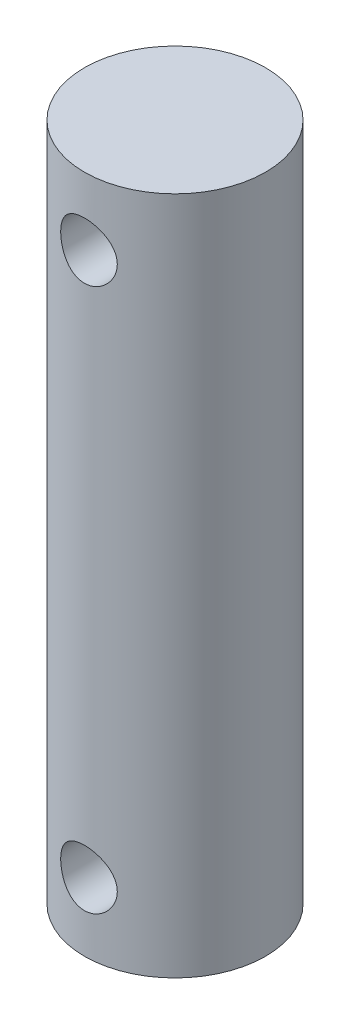
ISO-10303-21;
HEADER;
FILE_DESCRIPTION(('STEP AP214'),'2;1');
FILE_NAME('part.step','',(''),(''),'','','');
FILE_SCHEMA(('AUTOMOTIVE_DESIGN { 1 0 10303 214 1 1 1 1 }'));
ENDSEC;
DATA;
#1=APPLICATION_CONTEXT('core data for automotive mechanical design processes');
#2=APPLICATION_PROTOCOL_DEFINITION('international standard','automotive_design',2000,#1);
#3=PRODUCT_CONTEXT('',#1,'mechanical');
#4=PRODUCT('Part','Part','',(#3));
#5=PRODUCT_RELATED_PRODUCT_CATEGORY('part','',(#4));
#6=PRODUCT_DEFINITION_FORMATION('','',#4);
#7=PRODUCT_DEFINITION_CONTEXT('part definition',#1,'design');
#8=PRODUCT_DEFINITION('design','',#6,#7);
#9=PRODUCT_DEFINITION_SHAPE('','',#8);
#10=(LENGTH_UNIT() NAMED_UNIT(*) SI_UNIT(.MILLI.,.METRE.));
#11=(NAMED_UNIT(*) PLANE_ANGLE_UNIT() SI_UNIT($,.RADIAN.));
#12=(NAMED_UNIT(*) SI_UNIT($,.STERADIAN.) SOLID_ANGLE_UNIT());
#13=UNCERTAINTY_MEASURE_WITH_UNIT(LENGTH_MEASURE(1.E-05),#10,'distance_accuracy_value','');
#14=(GEOMETRIC_REPRESENTATION_CONTEXT(3) GLOBAL_UNCERTAINTY_ASSIGNED_CONTEXT((#13)) GLOBAL_UNIT_ASSIGNED_CONTEXT((#10,
#11,#12)) REPRESENTATION_CONTEXT('',''));
#15=CARTESIAN_POINT('',(0.,0.,0.));
#16=DIRECTION('',(0.,0.,1.));
#17=DIRECTION('',(1.,0.,0.));
#18=AXIS2_PLACEMENT_3D('',#15,#16,#17);
#19=CARTESIAN_POINT('',(0.,30.,0.));
#20=DIRECTION('',(0.,-1.,0.));
#21=DIRECTION('',(0.,0.,-1.));
#22=AXIS2_PLACEMENT_3D('',#19,#20,#21);
#23=CYLINDRICAL_SURFACE('',#22,8.);
#24=CARTESIAN_POINT('',(0.,26.5,-8.));
#25=CARTESIAN_POINT('',(-0.136878370349093,26.4999991068248,-7.9999993175598));
#26=CARTESIAN_POINT('',(-0.273766105005718,26.4887215461111,-7.99645389969682));
#27=CARTESIAN_POINT('',(-0.543538419176897,26.4440275169215,-7.98265788177613));
#28=CARTESIAN_POINT('',(-0.676422085451815,26.4106060372713,-7.97240576399719));
#29=CARTESIAN_POINT('',(-0.934257087301612,26.3228612576085,-7.94631631395819));
#30=CARTESIAN_POINT('',(-1.05922035397161,26.2685703106941,-7.9304876299805));
#31=CARTESIAN_POINT('',(-1.29826960469292,26.1407653646433,-7.89487938322185));
#32=CARTESIAN_POINT('',(-1.41235387088977,26.0672483364388,-7.8750991979981));
#33=CARTESIAN_POINT('',(-1.62993066990456,25.9006880159653,-7.83300427480565));
#34=CARTESIAN_POINT('',(-1.73304005631332,25.8071582298779,-7.81063431853978));
#35=CARTESIAN_POINT('',(-1.92239476407399,25.6042632151729,-7.76620092748417));
#36=CARTESIAN_POINT('',(-2.00863694579739,25.4948950450109,-7.74413755046915));
#37=CARTESIAN_POINT('',(-2.16388672966227,25.2601108723838,-7.70222289396344));
#38=CARTESIAN_POINT('',(-2.23241568300258,25.1343650449456,-7.68243976603591));
#39=CARTESIAN_POINT('',(-2.34719482153343,24.8724153700363,-7.64815603598469));
#40=CARTESIAN_POINT('',(-2.39345087543889,24.7362142884121,-7.63365404257377));
#41=CARTESIAN_POINT('',(-2.46096919860067,24.4615438450959,-7.61215213969001));
#42=CARTESIAN_POINT('',(-2.48294220015729,24.3232663127223,-7.60493945859016));
#43=CARTESIAN_POINT('',(-2.50349110073976,24.0448137621762,-7.59820110281901));
#44=CARTESIAN_POINT('',(-2.50207321991544,23.9046392583567,-7.59867338454668));
#45=CARTESIAN_POINT('',(-2.47643649465479,23.632251079462,-7.60706378150876));
#46=CARTESIAN_POINT('',(-2.45312115738766,23.4999417482769,-7.61468683491897));
#47=CARTESIAN_POINT('',(-2.38581626711252,23.2412156869253,-7.63604051304978));
#48=CARTESIAN_POINT('',(-2.34182451689101,23.1147995845824,-7.6497717868623));
#49=CARTESIAN_POINT('',(-2.23377749362554,22.8692961111347,-7.68202088028593));
#50=CARTESIAN_POINT('',(-2.16943851324164,22.750342778616,-7.70060569321649));
#51=CARTESIAN_POINT('',(-2.02272041475696,22.5246244642418,-7.7404371316014));
#52=CARTESIAN_POINT('',(-1.94033661043155,22.4178626594926,-7.76168444789102));
#53=CARTESIAN_POINT('',(-1.75543390836425,22.214450113166,-7.80563055600986));
#54=CARTESIAN_POINT('',(-1.65216914118563,22.1184808844406,-7.82835139211391));
#55=CARTESIAN_POINT('',(-1.43072881619106,21.9450562128406,-7.87183141519161));
#56=CARTESIAN_POINT('',(-1.31255215469804,21.8676021415616,-7.89259045676745));
#57=CARTESIAN_POINT('',(-1.06332922093091,21.7329446227975,-7.93002589780382));
#58=CARTESIAN_POINT('',(-0.932189813838561,21.6759037290721,-7.94666921296415));
#59=CARTESIAN_POINT('',(-0.661535955565289,21.5848939982969,-7.97375911657108));
#60=CARTESIAN_POINT('',(-0.522024061449216,21.5509181555232,-7.98420758650304));
#61=CARTESIAN_POINT('',(-0.244370314580689,21.508163914842,-7.99742778790027));
#62=CARTESIAN_POINT('',(-0.106383697577685,21.498462912813,-8.00048045790873));
#63=CARTESIAN_POINT('',(0.169260611465172,21.5019324532747,-7.99939599461967));
#64=CARTESIAN_POINT('',(0.306918348613018,21.5150996546452,-7.9952599116227));
#65=CARTESIAN_POINT('',(0.574438665951698,21.5631911852128,-7.98044727539523));
#66=CARTESIAN_POINT('',(0.704409956841874,21.597566535225,-7.96993586221374));
#67=CARTESIAN_POINT('',(0.956703857722754,21.6864287047334,-7.94360242758579));
#68=CARTESIAN_POINT('',(1.07902552089812,21.74091800805,-7.92777975028687));
#69=CARTESIAN_POINT('',(1.31586481334438,21.8699464330974,-7.89197085518848));
#70=CARTESIAN_POINT('',(1.43011947957558,21.9449419749936,-7.87189253635335));
#71=CARTESIAN_POINT('',(1.64473170192052,22.1123064202348,-7.82986820006859));
#72=CARTESIAN_POINT('',(1.7450854760879,22.2046800354893,-7.80792167695774));
#73=CARTESIAN_POINT('',(1.93317492583804,22.4085177801042,-7.76353989766283));
#74=CARTESIAN_POINT('',(2.02025304679063,22.5205933274784,-7.74111973412882));
#75=CARTESIAN_POINT('',(2.17442500490303,22.7582532327535,-7.69923894191212));
#76=CARTESIAN_POINT('',(2.24151915946859,22.883837376054,-7.67977826622621));
#77=CARTESIAN_POINT('',(2.35340166961085,23.144690345741,-7.64623564661738));
#78=CARTESIAN_POINT('',(2.39827639112025,23.2799192988714,-7.63213292713749));
#79=CARTESIAN_POINT('',(2.4644578863618,23.5565449864972,-7.6110234168862));
#80=CARTESIAN_POINT('',(2.48577362827989,23.6979393526871,-7.60401392602456));
#81=CARTESIAN_POINT('',(2.50358812316251,23.9760081751609,-7.59816585427753));
#82=CARTESIAN_POINT('',(2.50116559243271,24.1126069076948,-7.59897209200284));
#83=CARTESIAN_POINT('',(2.47417636257668,24.3833491698839,-7.60780180751807));
#84=CARTESIAN_POINT('',(2.44961069645024,24.5174928137735,-7.61582494863208));
#85=CARTESIAN_POINT('',(2.37975459827235,24.7775880791838,-7.6379362836678));
#86=CARTESIAN_POINT('',(2.33477284812017,24.9036308821867,-7.65193396380514));
#87=CARTESIAN_POINT('',(2.22560454669999,25.146480827068,-7.68439408509128));
#88=CARTESIAN_POINT('',(2.16141408888474,25.2632860841568,-7.70285743429343));
#89=CARTESIAN_POINT('',(2.01271350026987,25.4892919408796,-7.74306974067005));
#90=CARTESIAN_POINT('',(1.92750667048265,25.5980162590005,-7.76491897845913));
#91=CARTESIAN_POINT('',(1.7404179928096,25.799972656224,-7.8089799764242));
#92=CARTESIAN_POINT('',(1.63853168468878,25.8932005779821,-7.83119183213309));
#93=CARTESIAN_POINT('',(1.41697332564669,26.0645650767259,-7.87434543904947));
#94=CARTESIAN_POINT('',(1.29682914897477,26.1421094728999,-7.89522203461346));
#95=CARTESIAN_POINT('',(1.0445582760273,26.2757978302789,-7.93253538593756));
#96=CARTESIAN_POINT('',(0.912436315590895,26.3319502042837,-7.94897388631644));
#97=CARTESIAN_POINT('',(0.651495270747956,26.4171827352169,-7.97441301466941));
#98=CARTESIAN_POINT('',(0.523340674225092,26.4481497346107,-7.98392481612283));
#99=CARTESIAN_POINT('',(0.263459790880495,26.4895567199354,-7.99671800680967));
#100=CARTESIAN_POINT('',(0.131734232279349,26.500000859608,-8.00000065679286));
#101=CARTESIAN_POINT('',(0.,26.5,-8.));
#102=B_SPLINE_CURVE_WITH_KNOTS('',3,(#24,#25,#26,#27,#28,#29,#30,#31,#32,#33,#34,#35,#36,#37,
#38,#39,#40,#41,#42,#43,#44,#45,#46,#47,#48,#49,#50,#51,#52,#53,#54,#55,#56,#57,#58,#59,#60,#61,
#62,#63,#64,#65,#66,#67,#68,#69,#70,#71,#72,#73,#74,#75,#76,#77,#78,#79,#80,#81,#82,#83,#84,#85,
#86,#87,#88,#89,#90,#91,#92,#93,#94,#95,#96,#97,#98,#99,#100,#101),.UNSPECIFIED.,.T.,.F.,(4,2,2,
2,2,2,2,2,2,2,2,2,2,2,2,2,2,2,2,2,2,2,2,2,2,2,2,2,2,2,2,2,2,2,2,2,2,2,4),(0.,0.41015089886502,
0.820394646698132,1.23000495840487,1.63967984311678,2.06075644390316,2.48191134862552,
2.91347542494988,3.34492572559054,3.7633830033442,4.18172900590277,4.58353834844338,
4.98539039958126,5.39311285441091,5.80094132020717,6.22733494559201,6.65376014826606,
7.0835092137954,7.51312768989108,7.92615137096475,8.33911471298726,8.74181253445744,
9.14456010069,9.55712649476687,9.96980491418519,10.3988355742628,10.8278594196742,
11.2552023150671,11.6823824779468,12.0902440696666,12.4980866352126,12.8999582681244,
13.3019116867944,13.7195902803182,14.1373807476578,14.5688133627192,15.0000761335177,
15.3948927332218,15.7896294154519),.UNSPECIFIED.);
#103=CARTESIAN_POINT('',(0.,26.5,-8.));
#104=VERTEX_POINT('',#103);
#105=EDGE_CURVE('E10',#104,#104,#102,.T.);
#106=ORIENTED_EDGE('',*,*,#105,.T.);
#107=EDGE_LOOP('',(#106));
#108=FACE_BOUND('',#107,.T.);
#109=CARTESIAN_POINT('',(2.5,24.,7.59934207678533));
#110=CARTESIAN_POINT('',(2.49999907560094,23.8633059277813,7.59934291923872));
#111=CARTESIAN_POINT('',(2.48875077582989,23.7266024625936,7.60307063010085));
#112=CARTESIAN_POINT('',(2.44418350802654,23.4572116782444,7.61751277997754));
#113=CARTESIAN_POINT('',(2.4108585756503,23.3245254545357,7.62822910706272));
#114=CARTESIAN_POINT('',(2.32339576447118,23.067110196136,7.65531877671919));
#115=CARTESIAN_POINT('',(2.26929471473354,22.9423675337886,7.67168210388634));
#116=CARTESIAN_POINT('',(2.14193828346314,22.703694608272,7.70820812437377));
#117=CARTESIAN_POINT('',(2.06867951811264,22.5897662600798,7.72837148871681));
#118=CARTESIAN_POINT('',(1.90239214124459,22.372042265013,7.7710025533724));
#119=CARTESIAN_POINT('',(1.8088187994408,22.268672781128,7.79352246769561));
#120=CARTESIAN_POINT('',(1.60572409291099,22.0788079735816,7.83788491720671));
#121=CARTESIAN_POINT('',(1.49620050503713,21.9923150061103,7.85972735745255));
#122=CARTESIAN_POINT('',(1.26125182498672,21.8367778739775,7.90087106780156));
#123=CARTESIAN_POINT('',(1.13552311304019,21.7681725923371,7.9201036912556));
#124=CARTESIAN_POINT('',(0.873608465706806,21.6532479002889,7.95325103666038));
#125=CARTESIAN_POINT('',(0.737424996974103,21.6069232517008,7.9671670083984));
#126=CARTESIAN_POINT('',(0.462928713932197,21.5392977438059,7.98774351641724));
#127=CARTESIAN_POINT('',(0.324811430936433,21.5172685004243,7.99461477968283));
#128=CARTESIAN_POINT('',(0.0466816279690395,21.496551307125,8.00107191752033));
#129=CARTESIAN_POINT('',(-0.0933304539461723,21.4978580512823,8.00065944820141));
#130=CARTESIAN_POINT('',(-0.366148960709462,21.5232965831719,7.99274232265063));
#131=CARTESIAN_POINT('',(-0.499037268628064,21.546638767026,7.98548301944274));
#132=CARTESIAN_POINT('',(-0.75890612669556,21.614189980086,7.9649896512175));
#133=CARTESIAN_POINT('',(-0.88588629096247,21.6584003701733,7.95175519654419));
#134=CARTESIAN_POINT('',(-1.13215620630948,21.7669403781496,7.92046919458913));
#135=CARTESIAN_POINT('',(-1.25133281124535,21.8315096171255,7.90236067233341));
#136=CARTESIAN_POINT('',(-1.47740502230436,21.9787421994097,7.86323445907697));
#137=CARTESIAN_POINT('',(-1.58429751241882,22.0614101182777,7.84221603291309));
#138=CARTESIAN_POINT('',(-1.78747539690657,22.2465472696004,7.79847341467064));
#139=CARTESIAN_POINT('',(-1.88313309818382,22.3496981376742,7.77571463969686));
#140=CARTESIAN_POINT('',(-2.05597948519529,22.5707902036571,7.73181230889308));
#141=CARTESIAN_POINT('',(-2.13316599552377,22.6887331411807,7.71066894351396));
#142=CARTESIAN_POINT('',(-2.26760930038169,22.9378349376951,7.6722169326579));
#143=CARTESIAN_POINT('',(-2.32463361399527,23.0691268179819,7.65495380588195));
#144=CARTESIAN_POINT('',(-2.41556691891091,23.340118983684,7.62675090557699));
#145=CARTESIAN_POINT('',(-2.44948421530003,23.4798162283887,7.61580886035023));
#146=CARTESIAN_POINT('',(-2.4920297037281,23.7576399051543,7.60199126814082));
#147=CARTESIAN_POINT('',(-2.50161908707794,23.8956039924703,7.59880932787512));
#148=CARTESIAN_POINT('',(-2.49793488996242,24.1711794829903,7.6000215491985));
#149=CARTESIAN_POINT('',(-2.48466484222813,24.3087909373993,7.60441454014633));
#150=CARTESIAN_POINT('',(-2.43649747026382,24.5756165933048,7.61997914967833));
#151=CARTESIAN_POINT('',(-2.40223662321101,24.7049585481484,7.63095108204023));
#152=CARTESIAN_POINT('',(-2.31380747322029,24.9560435839917,7.65822574662762));
#153=CARTESIAN_POINT('',(-2.25963592342302,25.0777854218423,7.67452934824624));
#154=CARTESIAN_POINT('',(-2.13115021311757,25.3140782195436,7.71121079306468));
#155=CARTESIAN_POINT('',(-2.05630294977117,25.4283228311856,7.73169206979508));
#156=CARTESIAN_POINT('',(-1.8892128173596,25.6429806927238,7.77420697945615));
#157=CARTESIAN_POINT('',(-1.79696542938156,25.7433903378507,7.79624101471394));
#158=CARTESIAN_POINT('',(-1.59314589550721,25.9318207318256,7.84048375125371));
#159=CARTESIAN_POINT('',(-1.48093129957704,26.0191555722797,7.86266184571362));
#160=CARTESIAN_POINT('',(-1.24290309130279,26.1737820866425,7.90378119687353));
#161=CARTESIAN_POINT('',(-1.11709010221725,26.2410746786221,7.92272260181891));
#162=CARTESIAN_POINT('',(-0.856211046663665,26.3530611249434,7.95512623857025));
#163=CARTESIAN_POINT('',(-0.721220368567513,26.3979185756874,7.968627991224));
#164=CARTESIAN_POINT('',(-0.445114508112781,26.4641450771794,7.98880485297152));
#165=CARTESIAN_POINT('',(-0.304001256680715,26.485521478167,7.99548209828555));
#166=CARTESIAN_POINT('',(-0.0259698732978004,26.5035820034992,8.00111606808923));
#167=CARTESIAN_POINT('',(0.110878383893042,26.5012569003415,8.0003825881478));
#168=CARTESIAN_POINT('',(0.382146443846494,26.4743763779026,7.99201956162097));
#169=CARTESIAN_POINT('',(0.516566404359135,26.4498224080161,7.98439046465238));
#170=CARTESIAN_POINT('',(0.777510236961581,26.3798119815555,7.96319141689591));
#171=CARTESIAN_POINT('',(0.904111836898961,26.3346207843093,7.9496969592041));
#172=CARTESIAN_POINT('',(1.14799685100018,26.224858345583,7.918158911759));
#173=CARTESIAN_POINT('',(1.26527866254896,26.1602837800531,7.90011454182716));
#174=CARTESIAN_POINT('',(1.49152338993938,26.0110544833111,7.86059793766752));
#175=CARTESIAN_POINT('',(1.60006921410622,25.9257929550721,7.83903019501924));
#176=CARTESIAN_POINT('',(1.80164158279864,25.7386802211131,7.79517473094122));
#177=CARTESIAN_POINT('',(1.89466346700832,25.6368240517212,7.77288679569653));
#178=CARTESIAN_POINT('',(2.06565731822505,25.4153685603178,7.72923785154876));
#179=CARTESIAN_POINT('',(2.14302855989422,25.2952931937668,7.70793201726912));
#180=CARTESIAN_POINT('',(2.27640941497043,25.0432037594617,7.66960250559062));
#181=CARTESIAN_POINT('',(2.33242766807092,24.9111945470995,7.65257709722773));
#182=CARTESIAN_POINT('',(2.41742360871585,24.6505547653707,7.62613120880655));
#183=CARTESIAN_POINT('',(2.44829879675747,24.5225949050969,7.61618630087498));
#184=CARTESIAN_POINT('',(2.48958491632199,24.263092335807,7.60279212964797));
#185=CARTESIAN_POINT('',(2.50000088961557,24.131550517597,7.59934126603196));
#186=CARTESIAN_POINT('',(2.5,24.,7.59934207678533));
#187=B_SPLINE_CURVE_WITH_KNOTS('',3,(#109,#110,#111,#112,#113,#114,#115,#116,#117,#118,#119,
#120,#121,#122,#123,#124,#125,#126,#127,#128,#129,#130,#131,#132,#133,#134,#135,#136,#137,#138,
#139,#140,#141,#142,#143,#144,#145,#146,#147,#148,#149,#150,#151,#152,#153,#154,#155,#156,#157,
#158,#159,#160,#161,#162,#163,#164,#165,#166,#167,#168,#169,#170,#171,#172,#173,#174,#175,#176,
#177,#178,#179,#180,#181,#182,#183,#184,#185,#186),.UNSPECIFIED.,.T.,.F.,(4,2,2,2,2,2,2,2,2,2,2,
2,2,2,2,2,2,2,2,2,2,2,2,2,2,2,2,2,2,2,2,2,2,2,2,2,2,2,4),(0.,0.409596275096981,
0.819303254119471,1.22828728823716,1.6373436098499,2.05914161101677,2.48099845882246,
2.91239643927466,3.34369294835844,3.76167445671067,4.17956092943549,4.58301965939501,
4.98650470380186,5.39492809216818,5.80345485426375,6.22900677874668,6.65460879707552,
7.08496941871143,7.51517527910369,7.92809866580735,8.34095824443042,8.7418794409359,
9.14286604511284,9.55535226624085,9.96794576028624,10.3976387562789,10.8273120663904,
11.2538047858686,11.6801639628603,12.0887760488391,12.4973614938948,12.9008369303438,
13.3043815982817,13.7216138621529,14.1389711554924,14.5701559100827,15.0011660161251,
15.3954470874764,15.7896309838242),.UNSPECIFIED.);
#188=CARTESIAN_POINT('',(2.5,24.,7.59934207678533));
#189=VERTEX_POINT('',#188);
#190=EDGE_CURVE('E48',#189,#189,#187,.T.);
#191=ORIENTED_EDGE('',*,*,#190,.T.);
#192=EDGE_LOOP('',(#191));
#193=FACE_BOUND('',#192,.T.);
#194=CARTESIAN_POINT('',(0.,-21.5,-8.));
#195=CARTESIAN_POINT('',(-0.136878370349093,-21.5000008931752,-7.9999993175598));
#196=CARTESIAN_POINT('',(-0.273766105005718,-21.5112784538889,-7.99645389969682));
#197=CARTESIAN_POINT('',(-0.543538419176897,-21.5559724830785,-7.98265788177613));
#198=CARTESIAN_POINT('',(-0.676422085451815,-21.5893939627287,-7.97240576399719));
#199=CARTESIAN_POINT('',(-0.934257087301612,-21.6771387423915,-7.94631631395819));
#200=CARTESIAN_POINT('',(-1.05922035397161,-21.7314296893059,-7.9304876299805));
#201=CARTESIAN_POINT('',(-1.29826960469292,-21.8592346353567,-7.89487938322185));
#202=CARTESIAN_POINT('',(-1.41235387088977,-21.9327516635612,-7.8750991979981));
#203=CARTESIAN_POINT('',(-1.62993066990456,-22.0993119840347,-7.83300427480565));
#204=CARTESIAN_POINT('',(-1.73304005631332,-22.1928417701221,-7.81063431853978));
#205=CARTESIAN_POINT('',(-1.92239476407399,-22.3957367848271,-7.76620092748417));
#206=CARTESIAN_POINT('',(-2.00863694579739,-22.5051049549891,-7.74413755046915));
#207=CARTESIAN_POINT('',(-2.16388672966227,-22.7398891276162,-7.70222289396344));
#208=CARTESIAN_POINT('',(-2.23241568300257,-22.8656349550544,-7.68243976603591));
#209=CARTESIAN_POINT('',(-2.34719482153343,-23.1275846299637,-7.64815603598469));
#210=CARTESIAN_POINT('',(-2.39345087543889,-23.2637857115879,-7.63365404257377));
#211=CARTESIAN_POINT('',(-2.46096919860067,-23.5384561549041,-7.61215213969001));
#212=CARTESIAN_POINT('',(-2.48294220015729,-23.6767336872777,-7.60493945859016));
#213=CARTESIAN_POINT('',(-2.50349110073976,-23.9551862378238,-7.59820110281901));
#214=CARTESIAN_POINT('',(-2.50207321991544,-24.0953607416433,-7.59867338454668));
#215=CARTESIAN_POINT('',(-2.47643649465479,-24.367748920538,-7.60706378150876));
#216=CARTESIAN_POINT('',(-2.45312115738766,-24.5000582517231,-7.61468683491897));
#217=CARTESIAN_POINT('',(-2.38581626711252,-24.7587843130747,-7.63604051304978));
#218=CARTESIAN_POINT('',(-2.34182451689101,-24.8852004154176,-7.6497717868623));
#219=CARTESIAN_POINT('',(-2.23377749362554,-25.1307038888653,-7.68202088028593));
#220=CARTESIAN_POINT('',(-2.16943851324164,-25.249657221384,-7.70060569321649));
#221=CARTESIAN_POINT('',(-2.02272041475696,-25.4753755357583,-7.7404371316014));
#222=CARTESIAN_POINT('',(-1.94033661043155,-25.5821373405074,-7.76168444789102));
#223=CARTESIAN_POINT('',(-1.75543390836425,-25.785549886834,-7.80563055600986));
#224=CARTESIAN_POINT('',(-1.65216914118563,-25.8815191155594,-7.82835139211391));
#225=CARTESIAN_POINT('',(-1.43072881619106,-26.0549437871594,-7.87183141519161));
#226=CARTESIAN_POINT('',(-1.31255215469804,-26.1323978584384,-7.89259045676745));
#227=CARTESIAN_POINT('',(-1.06332922093091,-26.2670553772026,-7.93002589780382));
#228=CARTESIAN_POINT('',(-0.932189813838561,-26.3240962709279,-7.94666921296415));
#229=CARTESIAN_POINT('',(-0.661535955565289,-26.4151060017031,-7.97375911657108));
#230=CARTESIAN_POINT('',(-0.522024061449216,-26.4490818444768,-7.98420758650304));
#231=CARTESIAN_POINT('',(-0.244370314580689,-26.491836085158,-7.99742778790027));
#232=CARTESIAN_POINT('',(-0.106383697577685,-26.5015370871871,-8.00048045790873));
#233=CARTESIAN_POINT('',(0.169260611465172,-26.4980675467253,-7.99939599461967));
#234=CARTESIAN_POINT('',(0.306918348613018,-26.4849003453548,-7.9952599116227));
#235=CARTESIAN_POINT('',(0.574438665951697,-26.4368088147872,-7.98044727539523));
#236=CARTESIAN_POINT('',(0.704409956841873,-26.402433464775,-7.96993586221374));
#237=CARTESIAN_POINT('',(0.956703857722753,-26.3135712952666,-7.94360242758579));
#238=CARTESIAN_POINT('',(1.07902552089812,-26.25908199195,-7.92777975028687));
#239=CARTESIAN_POINT('',(1.31586481334438,-26.1300535669026,-7.89197085518848));
#240=CARTESIAN_POINT('',(1.43011947957558,-26.0550580250064,-7.87189253635335));
#241=CARTESIAN_POINT('',(1.64473170192052,-25.8876935797652,-7.82986820006859));
#242=CARTESIAN_POINT('',(1.7450854760879,-25.7953199645107,-7.80792167695774));
#243=CARTESIAN_POINT('',(1.93317492583804,-25.5914822198958,-7.76353989766283));
#244=CARTESIAN_POINT('',(2.02025304679062,-25.4794066725216,-7.74111973412883));
#245=CARTESIAN_POINT('',(2.17442500490303,-25.2417467672465,-7.69923894191212));
#246=CARTESIAN_POINT('',(2.24151915946859,-25.116162623946,-7.67977826622621));
#247=CARTESIAN_POINT('',(2.35340166961084,-24.855309654259,-7.64623564661738));
#248=CARTESIAN_POINT('',(2.39827639112025,-24.7200807011286,-7.63213292713749));
#249=CARTESIAN_POINT('',(2.4644578863618,-24.4434550135028,-7.6110234168862));
#250=CARTESIAN_POINT('',(2.48577362827989,-24.3020606473129,-7.60401392602456));
#251=CARTESIAN_POINT('',(2.50358812316251,-24.0239918248391,-7.59816585427753));
#252=CARTESIAN_POINT('',(2.50116559243271,-23.8873930923052,-7.59897209200284));
#253=CARTESIAN_POINT('',(2.47417636257668,-23.6166508301161,-7.60780180751807));
#254=CARTESIAN_POINT('',(2.44961069645024,-23.4825071862265,-7.61582494863208));
#255=CARTESIAN_POINT('',(2.37975459827235,-23.2224119208162,-7.6379362836678));
#256=CARTESIAN_POINT('',(2.33477284812016,-23.0963691178133,-7.65193396380514));
#257=CARTESIAN_POINT('',(2.22560454669999,-22.853519172932,-7.68439408509128));
#258=CARTESIAN_POINT('',(2.16141408888474,-22.7367139158432,-7.70285743429343));
#259=CARTESIAN_POINT('',(2.01271350026987,-22.5107080591204,-7.74306974067005));
#260=CARTESIAN_POINT('',(1.92750667048265,-22.4019837409995,-7.76491897845913));
#261=CARTESIAN_POINT('',(1.7404179928096,-22.200027343776,-7.8089799764242));
#262=CARTESIAN_POINT('',(1.63853168468878,-22.1067994220179,-7.83119183213309));
#263=CARTESIAN_POINT('',(1.41697332564669,-21.9354349232741,-7.87434543904947));
#264=CARTESIAN_POINT('',(1.29682914897477,-21.8578905271001,-7.89522203461346));
#265=CARTESIAN_POINT('',(1.0445582760273,-21.7242021697211,-7.93253538593756));
#266=CARTESIAN_POINT('',(0.912436315590895,-21.6680497957163,-7.94897388631644));
#267=CARTESIAN_POINT('',(0.651495270747956,-21.5828172647831,-7.97441301466941));
#268=CARTESIAN_POINT('',(0.523340674225092,-21.5518502653893,-7.98392481612283));
#269=CARTESIAN_POINT('',(0.263459790880495,-21.5104432800646,-7.99671800680967));
#270=CARTESIAN_POINT('',(0.131734232279349,-21.499999140392,-8.00000065679286));
#271=CARTESIAN_POINT('',(0.,-21.5,-8.));
#272=B_SPLINE_CURVE_WITH_KNOTS('',3,(#194,#195,#196,#197,#198,#199,#200,#201,#202,#203,#204,
#205,#206,#207,#208,#209,#210,#211,#212,#213,#214,#215,#216,#217,#218,#219,#220,#221,#222,#223,
#224,#225,#226,#227,#228,#229,#230,#231,#232,#233,#234,#235,#236,#237,#238,#239,#240,#241,#242,
#243,#244,#245,#246,#247,#248,#249,#250,#251,#252,#253,#254,#255,#256,#257,#258,#259,#260,#261,
#262,#263,#264,#265,#266,#267,#268,#269,#270,#271),.UNSPECIFIED.,.T.,.F.,(4,2,2,2,2,2,2,2,2,2,2,
2,2,2,2,2,2,2,2,2,2,2,2,2,2,2,2,2,2,2,2,2,2,2,2,2,2,2,4),(0.,0.41015089886502,0.820394646698132,
1.23000495840487,1.63967984311678,2.06075644390316,2.48191134862552,2.91347542494988,
3.34492572559054,3.7633830033442,4.18172900590276,4.58353834844338,4.98539039958126,
5.39311285441091,5.80094132020717,6.227334945592,6.65376014826606,7.0835092137954,
7.51312768989108,7.92615137096475,8.33911471298726,8.74181253445744,9.14456010069,
9.55712649476687,9.96980491418519,10.3988355742628,10.8278594196742,11.2552023150671,
11.6823824779468,12.0902440696666,12.4980866352126,12.8999582681244,13.3019116867944,
13.7195902803182,14.1373807476578,14.5688133627192,15.0000761335177,15.3948927332218,
15.7896294154519),.UNSPECIFIED.);
#273=CARTESIAN_POINT('',(0.,-21.5,-8.));
#274=VERTEX_POINT('',#273);
#275=EDGE_CURVE('E55',#274,#274,#272,.T.);
#276=ORIENTED_EDGE('',*,*,#275,.T.);
#277=EDGE_LOOP('',(#276));
#278=FACE_BOUND('',#277,.T.);
#279=CARTESIAN_POINT('',(2.5,-24.,7.59934207678533));
#280=CARTESIAN_POINT('',(2.49999907560094,-24.1366940722187,7.59934291923872));
#281=CARTESIAN_POINT('',(2.48875077582989,-24.2733975374064,7.60307063010085));
#282=CARTESIAN_POINT('',(2.44418350802654,-24.5427883217556,7.61751277997754));
#283=CARTESIAN_POINT('',(2.4108585756503,-24.6754745454643,7.62822910706272));
#284=CARTESIAN_POINT('',(2.32339576447118,-24.932889803864,7.65531877671919));
#285=CARTESIAN_POINT('',(2.26929471473354,-25.0576324662114,7.67168210388634));
#286=CARTESIAN_POINT('',(2.14193828346314,-25.296305391728,7.70820812437377));
#287=CARTESIAN_POINT('',(2.06867951811264,-25.4102337399202,7.72837148871681));
#288=CARTESIAN_POINT('',(1.90239214124459,-25.627957734987,7.7710025533724));
#289=CARTESIAN_POINT('',(1.8088187994408,-25.731327218872,7.79352246769561));
#290=CARTESIAN_POINT('',(1.60572409291099,-25.9211920264184,7.83788491720671));
#291=CARTESIAN_POINT('',(1.49620050503713,-26.0076849938897,7.85972735745255));
#292=CARTESIAN_POINT('',(1.26125182498672,-26.1632221260225,7.90087106780156));
#293=CARTESIAN_POINT('',(1.13552311304019,-26.2318274076629,7.9201036912556));
#294=CARTESIAN_POINT('',(0.873608465706806,-26.3467520997111,7.95325103666038));
#295=CARTESIAN_POINT('',(0.737424996974103,-26.3930767482992,7.9671670083984));
#296=CARTESIAN_POINT('',(0.462928713932197,-26.4607022561941,7.98774351641724));
#297=CARTESIAN_POINT('',(0.324811430936433,-26.4827314995757,7.99461477968283));
#298=CARTESIAN_POINT('',(0.0466816279690395,-26.503448692875,8.00107191752033));
#299=CARTESIAN_POINT('',(-0.0933304539461723,-26.5021419487177,8.00065944820141));
#300=CARTESIAN_POINT('',(-0.366148960709462,-26.4767034168281,7.99274232265063));
#301=CARTESIAN_POINT('',(-0.499037268628064,-26.453361232974,7.98548301944274));
#302=CARTESIAN_POINT('',(-0.75890612669556,-26.385810019914,7.9649896512175));
#303=CARTESIAN_POINT('',(-0.88588629096247,-26.3415996298267,7.95175519654419));
#304=CARTESIAN_POINT('',(-1.13215620630948,-26.2330596218504,7.92046919458913));
#305=CARTESIAN_POINT('',(-1.25133281124535,-26.1684903828745,7.90236067233341));
#306=CARTESIAN_POINT('',(-1.47740502230436,-26.0212578005903,7.86323445907697));
#307=CARTESIAN_POINT('',(-1.58429751241882,-25.9385898817223,7.84221603291309));
#308=CARTESIAN_POINT('',(-1.78747539690657,-25.7534527303996,7.79847341467064));
#309=CARTESIAN_POINT('',(-1.88313309818382,-25.6503018623258,7.77571463969686));
#310=CARTESIAN_POINT('',(-2.05597948519529,-25.4292097963429,7.73181230889308));
#311=CARTESIAN_POINT('',(-2.13316599552377,-25.3112668588193,7.71066894351396));
#312=CARTESIAN_POINT('',(-2.26760930038169,-25.0621650623049,7.6722169326579));
#313=CARTESIAN_POINT('',(-2.32463361399527,-24.9308731820181,7.65495380588195));
#314=CARTESIAN_POINT('',(-2.41556691891091,-24.659881016316,7.62675090557699));
#315=CARTESIAN_POINT('',(-2.44948421530003,-24.5201837716113,7.61580886035023));
#316=CARTESIAN_POINT('',(-2.4920297037281,-24.2423600948457,7.60199126814082));
#317=CARTESIAN_POINT('',(-2.50161908707794,-24.1043960075297,7.59880932787512));
#318=CARTESIAN_POINT('',(-2.49793488996242,-23.8288205170097,7.6000215491985));
#319=CARTESIAN_POINT('',(-2.48466484222813,-23.6912090626007,7.60441454014633));
#320=CARTESIAN_POINT('',(-2.43649747026382,-23.4243834066952,7.61997914967833));
#321=CARTESIAN_POINT('',(-2.40223662321101,-23.2950414518516,7.63095108204023));
#322=CARTESIAN_POINT('',(-2.31380747322029,-23.0439564160083,7.65822574662762));
#323=CARTESIAN_POINT('',(-2.25963592342302,-22.9222145781577,7.67452934824624));
#324=CARTESIAN_POINT('',(-2.13115021311757,-22.6859217804564,7.71121079306468));
#325=CARTESIAN_POINT('',(-2.05630294977117,-22.5716771688144,7.73169206979508));
#326=CARTESIAN_POINT('',(-1.8892128173596,-22.3570193072762,7.77420697945615));
#327=CARTESIAN_POINT('',(-1.79696542938156,-22.2566096621493,7.79624101471394));
#328=CARTESIAN_POINT('',(-1.59314589550721,-22.0681792681744,7.84048375125371));
#329=CARTESIAN_POINT('',(-1.48093129957704,-21.9808444277203,7.86266184571362));
#330=CARTESIAN_POINT('',(-1.24290309130279,-21.8262179133575,7.90378119687353));
#331=CARTESIAN_POINT('',(-1.11709010221725,-21.7589253213779,7.92272260181891));
#332=CARTESIAN_POINT('',(-0.856211046663665,-21.6469388750566,7.95512623857025));
#333=CARTESIAN_POINT('',(-0.721220368567513,-21.6020814243126,7.968627991224));
#334=CARTESIAN_POINT('',(-0.445114508112781,-21.5358549228206,7.98880485297152));
#335=CARTESIAN_POINT('',(-0.304001256680715,-21.514478521833,7.99548209828555));
#336=CARTESIAN_POINT('',(-0.0259698732978004,-21.4964179965008,8.00111606808923));
#337=CARTESIAN_POINT('',(0.110878383893042,-21.4987430996585,8.0003825881478));
#338=CARTESIAN_POINT('',(0.382146443846494,-21.5256236220974,7.99201956162097));
#339=CARTESIAN_POINT('',(0.516566404359135,-21.5501775919839,7.98439046465238));
#340=CARTESIAN_POINT('',(0.777510236961581,-21.6201880184446,7.96319141689591));
#341=CARTESIAN_POINT('',(0.904111836898961,-21.6653792156907,7.9496969592041));
#342=CARTESIAN_POINT('',(1.14799685100018,-21.775141654417,7.918158911759));
#343=CARTESIAN_POINT('',(1.26527866254896,-21.8397162199469,7.90011454182716));
#344=CARTESIAN_POINT('',(1.49152338993938,-21.9889455166889,7.86059793766752));
#345=CARTESIAN_POINT('',(1.60006921410622,-22.0742070449279,7.83903019501924));
#346=CARTESIAN_POINT('',(1.80164158279864,-22.2613197788869,7.79517473094122));
#347=CARTESIAN_POINT('',(1.89466346700832,-22.3631759482788,7.77288679569653));
#348=CARTESIAN_POINT('',(2.06565731822505,-22.5846314396822,7.72923785154876));
#349=CARTESIAN_POINT('',(2.14302855989422,-22.7047068062331,7.70793201726912));
#350=CARTESIAN_POINT('',(2.27640941497043,-22.9567962405383,7.66960250559062));
#351=CARTESIAN_POINT('',(2.33242766807092,-23.0888054529005,7.65257709722773));
#352=CARTESIAN_POINT('',(2.41742360871585,-23.3494452346293,7.62613120880655));
#353=CARTESIAN_POINT('',(2.44829879675747,-23.4774050949031,7.61618630087498));
#354=CARTESIAN_POINT('',(2.48958491632199,-23.736907664193,7.60279212964797));
#355=CARTESIAN_POINT('',(2.50000088961557,-23.868449482403,7.59934126603196));
#356=CARTESIAN_POINT('',(2.5,-24.,7.59934207678533));
#357=B_SPLINE_CURVE_WITH_KNOTS('',3,(#279,#280,#281,#282,#283,#284,#285,#286,#287,#288,#289,
#290,#291,#292,#293,#294,#295,#296,#297,#298,#299,#300,#301,#302,#303,#304,#305,#306,#307,#308,
#309,#310,#311,#312,#313,#314,#315,#316,#317,#318,#319,#320,#321,#322,#323,#324,#325,#326,#327,
#328,#329,#330,#331,#332,#333,#334,#335,#336,#337,#338,#339,#340,#341,#342,#343,#344,#345,#346,
#347,#348,#349,#350,#351,#352,#353,#354,#355,#356),.UNSPECIFIED.,.T.,.F.,(4,2,2,2,2,2,2,2,2,2,2,
2,2,2,2,2,2,2,2,2,2,2,2,2,2,2,2,2,2,2,2,2,2,2,2,2,2,2,4),(0.,0.409596275096981,
0.819303254119471,1.22828728823716,1.6373436098499,2.05914161101677,2.48099845882246,
2.91239643927466,3.34369294835844,3.76167445671067,4.17956092943549,4.58301965939501,
4.98650470380186,5.39492809216818,5.80345485426375,6.22900677874668,6.65460879707552,
7.08496941871143,7.51517527910369,7.92809866580735,8.34095824443042,8.7418794409359,
9.14286604511284,9.55535226624085,9.96794576028624,10.3976387562789,10.8273120663904,
11.2538047858686,11.6801639628603,12.0887760488391,12.4973614938948,12.9008369303438,
13.3043815982817,13.7216138621529,14.1389711554924,14.5701559100827,15.0011660161251,
15.3954470874764,15.7896309838242),.UNSPECIFIED.);
#358=CARTESIAN_POINT('',(2.5,-24.,7.59934207678533));
#359=VERTEX_POINT('',#358);
#360=EDGE_CURVE('E57',#359,#359,#357,.T.);
#361=ORIENTED_EDGE('',*,*,#360,.T.);
#362=EDGE_LOOP('',(#361));
#363=FACE_BOUND('',#362,.T.);
#364=CARTESIAN_POINT('',(0.,30.,0.));
#365=DIRECTION('',(0.,1.,0.));
#366=DIRECTION('',(0.,0.,1.));
#367=AXIS2_PLACEMENT_3D('',#364,#365,#366);
#368=CIRCLE('',#367,8.);
#369=CARTESIAN_POINT('',(0.,30.,8.));
#370=VERTEX_POINT('',#369);
#371=EDGE_CURVE('E83',#370,#370,#368,.T.);
#372=ORIENTED_EDGE('',*,*,#371,.F.);
#373=EDGE_LOOP('',(#372));
#374=FACE_BOUND('',#373,.T.);
#375=CARTESIAN_POINT('',(0.,-30.,0.));
#376=DIRECTION('',(0.,1.,0.));
#377=DIRECTION('',(0.,0.,1.));
#378=AXIS2_PLACEMENT_3D('',#375,#376,#377);
#379=CIRCLE('',#378,8.);
#380=CARTESIAN_POINT('',(0.,-30.,8.));
#381=VERTEX_POINT('',#380);
#382=EDGE_CURVE('E84',#381,#381,#379,.T.);
#383=ORIENTED_EDGE('',*,*,#382,.T.);
#384=EDGE_LOOP('',(#383));
#385=FACE_BOUND('',#384,.T.);
#386=ADVANCED_FACE('F40',(#108,#193,#278,#363,#374,#385),#23,.T.);
#387=CARTESIAN_POINT('',(0.,30.,0.));
#388=DIRECTION('',(0.,1.,0.));
#389=DIRECTION('',(0.,0.,1.));
#390=AXIS2_PLACEMENT_3D('',#387,#388,#389);
#391=PLANE('',#390);
#392=ORIENTED_EDGE('',*,*,#371,.T.);
#393=EDGE_LOOP('',(#392));
#394=FACE_BOUND('',#393,.T.);
#395=ADVANCED_FACE('F76',(#394),#391,.T.);
#396=CARTESIAN_POINT('',(0.,-30.,0.));
#397=DIRECTION('',(0.,1.,0.));
#398=DIRECTION('',(0.,0.,1.));
#399=AXIS2_PLACEMENT_3D('',#396,#397,#398);
#400=PLANE('',#399);
#401=ORIENTED_EDGE('',*,*,#382,.F.);
#402=EDGE_LOOP('',(#401));
#403=FACE_BOUND('',#402,.T.);
#404=ADVANCED_FACE('F73',(#403),#400,.F.);
#405=CARTESIAN_POINT('',(0.,-24.,-8.));
#406=DIRECTION('',(0.,0.,1.));
#407=DIRECTION('',(1.,0.,0.));
#408=AXIS2_PLACEMENT_3D('',#405,#406,#407);
#409=CYLINDRICAL_SURFACE('',#408,2.5);
#410=ORIENTED_EDGE('',*,*,#360,.F.);
#411=EDGE_LOOP('',(#410));
#412=FACE_BOUND('',#411,.T.);
#413=ORIENTED_EDGE('',*,*,#275,.F.);
#414=EDGE_LOOP('',(#413));
#415=FACE_BOUND('',#414,.T.);
#416=ADVANCED_FACE('F68',(#412,#415),#409,.F.);
#417=CARTESIAN_POINT('',(0.,24.,-8.));
#418=DIRECTION('',(0.,0.,1.));
#419=DIRECTION('',(1.,0.,0.));
#420=AXIS2_PLACEMENT_3D('',#417,#418,#419);
#421=CYLINDRICAL_SURFACE('',#420,2.5);
#422=ORIENTED_EDGE('',*,*,#190,.F.);
#423=EDGE_LOOP('',(#422));
#424=FACE_BOUND('',#423,.T.);
#425=ORIENTED_EDGE('',*,*,#105,.F.);
#426=EDGE_LOOP('',(#425));
#427=FACE_BOUND('',#426,.T.);
#428=ADVANCED_FACE('F66',(#424,#427),#421,.F.);
#429=CLOSED_SHELL('',(#386,#395,#404,#416,#428));
#430=MANIFOLD_SOLID_BREP('B2',#429);
#431=ADVANCED_BREP_SHAPE_REPRESENTATION('',(#18,#430),#14);
#432=SHAPE_DEFINITION_REPRESENTATION(#9,#431);
ENDSEC;
END-ISO-10303-21;
